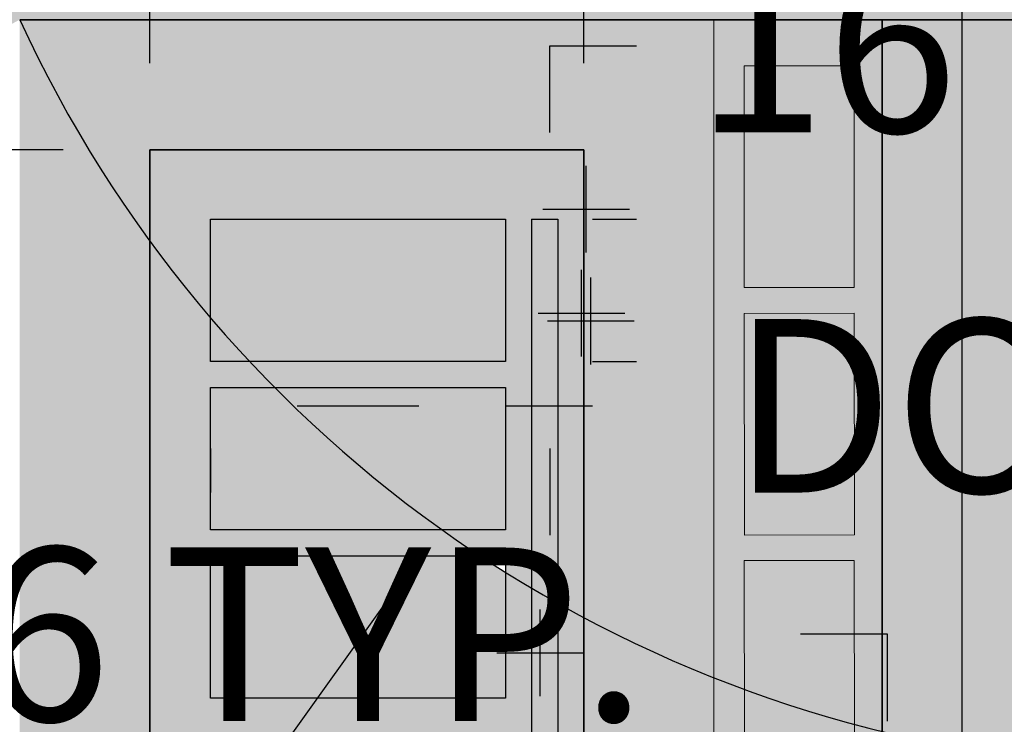
# Model space of a CAD drawing. Units: millimetres. Extents: x 130 to 1021, y 147 to 699.
# Tile 5 of 40: x 367 to 481, y 313 to 394. Entities that reach past the tile are written whole.
import ezdxf

# ---------------------------------------------------------------- set-up
doc = ezdxf.new("R2010")
doc.units = ezdxf.units.MM
doc.header["$MEASUREMENT"] = 0
for name, color, linetype, lineweight in [('A-ANNO-DIMS', 2, 'Continuous', 18), ('A-DOOR', 3, 'Continuous', 25), ('A-ELEV', 7, 'Continuous', 35), ('A-ELEV-PATT', 9, 'Continuous', 13), ('A-GLAZ', 4, 'Continuous', 18)]:
    doc.layers.add(name, color=color, linetype=linetype, lineweight=lineweight)
doc.styles.get("Standard").update_dxf_attribs({"font": 'arial.ttf'})
doc.dimstyles.get("Standard").update_dxf_attribs({"dimtxt": 20, "dimasz": 10, "dimexe": 10, "dimexo": 10, "dimgap": 5, "dimtad": 0, "dimtih": 1, "dimtoh": 1, "dimdec": 0, "dimzin": 0, "dimdsep": 46, "dimtxsty": 'Standard', "dimcen": 5, "dimadec": 0, "dimazin": 0, "dimtfac": 1, "dimtdec": 0, "dimtofl": 0, "dimtmove": 0, "dimatfit": 3, "dimfxl": 1, "dimtolj": 1, "dimtzin": 0, "dimarcsym": 0})

# ---------------------------------------------------------------- blocks, each defined once
blk = doc.blocks.new('DOOR-PANEL')
for p, q in [((0, 16.4), (34, 16.4)), ((0, 0), (0, 16.4)), ((34, 16.4), (34, 0)), ((34, 0), (0, 0))]:
    blk.add_line(p, q)
blk = doc.blocks.new('WIN-SIDELIGHT-PANE')
for p, q in [((0, 25.55), (12.68, 25.55)), ((0, 0), (0, 25.55)), ((12.68, 25.55), (12.68, 0)), ((12.68, 0), (0, 0))]:
    blk.add_line(p, q)
blk = doc.blocks.new('*D7')
at = {"layer": 'A-ANNO-DIMS', "color": 0, "lineweight": -2, "transparency": 16777216}
for p, q in [((399.37, 349.45), (413.37, 349.45)), ((423.37, 349.45), (433.37, 349.45)), ((389.37, 344.55), (389.37, 339.45)), ((423.37, 344.55), (423.37, 339.45))]:
    blk.add_line(p, q, dxfattribs=at)
at = {"layer": 'A-ANNO-DIMS', "color": 0, "transparency": 16777216}
for points in [[(399.37, 351.11), (399.37, 347.78), (389.37, 349.45)], [(413.37, 351.11), (413.37, 347.78), (423.37, 349.45)]]:
    blk.add_solid(points, dxfattribs=at)
at = {"layer": 'Defpoints', "color": 0, "transparency": 16777216}
for p in [(389.37, 354.55), (423.37, 354.55), (423.37, 349.45)]:
    blk.add_point(p, dxfattribs=at)
at = {"layer": 'A-ANNO-DIMS', "color": 0, "transparency": 16777216, "insert": (582.04, 349.45), "char_height": 20, "attachment_point": 5}
blk.add_mtext('\\A1;DOOR PANEL 34 TYP.', dxfattribs=at)
blk = doc.blocks.new('*D8')
at = {"layer": 'A-ANNO-DIMS', "color": 0, "lineweight": -2, "transparency": 16777216}
for p, q in [((428.47, 380.95), (428.47, 390.95)), ((428.47, 390.95), (438.47, 390.95)), ((433.37, 370.95), (438.47, 370.95)), ((433.37, 354.55), (438.47, 354.55)), ((428.47, 344.55), (428.47, 334.55))]:
    blk.add_line(p, q, dxfattribs=at)
at = {"layer": 'A-ANNO-DIMS', "color": 0, "transparency": 16777216}
for points in [[(426.81, 380.95), (430.14, 380.95), (428.47, 370.95)], [(426.81, 344.55), (430.14, 344.55), (428.47, 354.55)]]:
    blk.add_solid(points, dxfattribs=at)
at = {"layer": 'Defpoints', "color": 0, "transparency": 16777216}
for p in [(423.37, 370.95), (428.47, 370.95), (423.37, 354.55)]:
    blk.add_point(p, dxfattribs=at)
at = {"layer": 'A-ANNO-DIMS', "color": 0, "transparency": 16777216, "insert": (491.21, 390.95), "char_height": 20, "attachment_point": 5}
blk.add_mtext('\\A1;16 TYP.', dxfattribs=at)
blk = doc.blocks.new('*D9')
at = {"layer": 'A-ANNO-DIMS', "color": 0, "lineweight": -2, "transparency": 16777216}
for p, q in [((467.37, 323.13), (457.37, 323.13)), ((467.37, 313.13), (467.37, 323.13)), ((473.55, 303.13), (477.38, 303.13)), ((473.57, 277.58), (477.4, 277.58)), ((467.41, 267.57), (467.42, 257.57))]:
    blk.add_line(p, q, dxfattribs=at)
at = {"layer": 'A-ANNO-DIMS', "color": 0, "transparency": 16777216}
for points in [[(469.04, 313.13), (465.71, 313.13), (467.38, 303.13)], [(469.08, 267.57), (465.75, 267.57), (467.4, 277.57)]]:
    blk.add_solid(points, dxfattribs=at)
at = {"layer": 'Defpoints', "color": 0, "transparency": 16777216}
for p in [(463.55, 303.12), (467.38, 303.13), (463.57, 277.57)]:
    blk.add_point(p, dxfattribs=at)
at = {"layer": 'A-ANNO-DIMS', "color": 0, "transparency": 16777216, "insert": (284.19, 323.13), "char_height": 20, "attachment_point": 5}
blk.add_mtext('\\A1;SIDELIGHT PANE 26 TYP.', dxfattribs=at)
blk = doc.blocks.new('*D11')
at = {"layer": 'A-ANNO-DIMS', "color": 0, "lineweight": -2, "transparency": 16777216}
for p, q in [((737.37, 648.7), (737.37, 149.74)), ((299.37, 566.95), (299.37, 149.74)), ((309.37, 159.74), (490.86, 159.74)), ((727.37, 159.74), (545.89, 159.74))]:
    blk.add_line(p, q, dxfattribs=at)
at = {"layer": 'A-ANNO-DIMS', "color": 0, "transparency": 16777216}
for points in [[(309.37, 161.41), (309.37, 158.07), (299.37, 159.74)], [(727.37, 161.41), (727.37, 158.07), (737.37, 159.74)]]:
    blk.add_solid(points, dxfattribs=at)
at = {"layer": 'Defpoints', "color": 0, "transparency": 16777216}
for p in [(737.37, 658.7), (299.37, 576.95), (737.37, 159.74)]:
    blk.add_point(p, dxfattribs=at)
at = {"layer": 'A-ANNO-DIMS', "color": 0, "transparency": 16777216, "insert": (518.37, 159.74), "char_height": 20, "attachment_point": 5}
blk.add_mtext('\\A1;438', dxfattribs=at)
blk = doc.blocks.new('*D12')
at = {"layer": 'A-ANNO-DIMS', "color": 0, "lineweight": -2, "transparency": 16777216}
for p, q in [((477.37, 661.95), (265.07, 661.95)), ((275.07, 651.95), (275.07, 438.2)), ((275.07, 194.04), (275.07, 407.78)), ((357.16, 184.04), (265.07, 184.04))]:
    blk.add_line(p, q, dxfattribs=at)
at = {"layer": 'A-ANNO-DIMS', "color": 0, "transparency": 16777216}
for points in [[(273.41, 651.95), (276.74, 651.95), (275.07, 661.95)], [(273.41, 194.04), (276.74, 194.04), (275.07, 184.04)]]:
    blk.add_solid(points, dxfattribs=at)
at = {"layer": 'Defpoints', "color": 0, "transparency": 16777216}
for p in [(275.07, 661.95), (487.37, 661.95), (367.16, 184.04)]:
    blk.add_point(p, dxfattribs=at)
at = {"layer": 'A-ANNO-DIMS', "color": 0, "transparency": 16777216, "insert": (275.07, 422.99), "char_height": 20, "attachment_point": 5}
blk.add_mtext('\\A1;477.9', dxfattribs=at)
blk = doc.blocks.new('*D18')
at = {"layer": 'A-ANNO-DIMS', "color": 0, "lineweight": -2, "transparency": 16777216}
for p, q in [((375.85, 490.22), (375.85, 696.25)), ((382.37, 388.95), (382.37, 696.25)), ((365.85, 686.25), (355.85, 686.25)), ((392.37, 686.25), (402.37, 686.25))]:
    blk.add_line(p, q, dxfattribs=at)
at = {"layer": 'A-ANNO-DIMS', "color": 0, "transparency": 16777216}
for points in [[(365.85, 687.91), (365.85, 684.58), (375.85, 686.25)], [(392.37, 687.91), (392.37, 684.58), (382.37, 686.25)]]:
    blk.add_solid(points, dxfattribs=at)
at = {"layer": 'Defpoints', "color": 0, "transparency": 16777216}
for p in [(382.37, 686.25), (375.85, 480.22), (382.37, 378.95)]:
    blk.add_point(p, dxfattribs=at)
at = {"layer": 'A-ANNO-DIMS', "color": 0, "transparency": 16777216, "insert": (441.13, 686.25), "char_height": 20, "attachment_point": 5}
blk.add_mtext('\\A1;6.524', dxfattribs=at)
blk = doc.blocks.new('*D19')
at = {"layer": 'A-ANNO-DIMS', "color": 0, "lineweight": -2, "transparency": 16777216}
for p, q in [((382.37, 388.95), (382.37, 696.25)), ((414.65, 510.88), (414.65, 696.25)), ((392.37, 686.25), (404.65, 686.25)), ((414.65, 686.25), (424.65, 686.25))]:
    blk.add_line(p, q, dxfattribs=at)
at = {"layer": 'A-ANNO-DIMS', "color": 0, "transparency": 16777216}
for points in [[(392.37, 687.91), (392.37, 684.58), (382.37, 686.25)], [(404.65, 687.91), (404.65, 684.58), (414.65, 686.25)]]:
    blk.add_solid(points, dxfattribs=at)
at = {"layer": 'Defpoints', "color": 0, "transparency": 16777216}
for p in [(414.65, 686.25), (414.65, 500.88), (382.37, 378.95)]:
    blk.add_point(p, dxfattribs=at)
at = {"layer": 'A-ANNO-DIMS', "color": 0, "transparency": 16777216, "insert": (463.41, 686.25), "char_height": 20, "attachment_point": 5}
blk.add_mtext('\\A1;32.28', dxfattribs=at)
blk = doc.blocks.new('*D20')
at = {"layer": 'A-ANNO-DIMS', "color": 0, "lineweight": -2, "transparency": 16777216}
for p, q in [((414.65, 510.88), (414.65, 696.25)), ((432.37, 388.95), (432.37, 696.25)), ((404.65, 686.25), (394.65, 686.25)), ((442.37, 686.25), (452.37, 686.25))]:
    blk.add_line(p, q, dxfattribs=at)
at = {"layer": 'A-ANNO-DIMS', "color": 0, "transparency": 16777216}
for points in [[(404.65, 687.91), (404.65, 684.58), (414.65, 686.25)], [(442.37, 687.91), (442.37, 684.58), (432.37, 686.25)]]:
    blk.add_solid(points, dxfattribs=at)
at = {"layer": 'Defpoints', "color": 0, "transparency": 16777216}
for p in [(432.37, 686.25), (414.65, 500.88), (432.37, 378.95)]:
    blk.add_point(p, dxfattribs=at)
at = {"layer": 'A-ANNO-DIMS', "color": 0, "transparency": 16777216, "insert": (490.08, 686.25), "char_height": 20, "attachment_point": 5}
blk.add_mtext('\\A1;17.72', dxfattribs=at)
blk = doc.blocks.new('*D21')
at = {"layer": 'A-ANNO-DIMS', "color": 0, "lineweight": -2, "transparency": 16777216}
for p, q in [((432.37, 388.95), (432.37, 696.25)), ((447.37, 656.95), (447.37, 696.25)), ((422.37, 686.25), (412.37, 686.25)), ((457.37, 686.25), (467.37, 686.25))]:
    blk.add_line(p, q, dxfattribs=at)
at = {"layer": 'A-ANNO-DIMS', "color": 0, "transparency": 16777216}
for points in [[(422.37, 687.91), (422.37, 684.58), (432.37, 686.25)], [(457.37, 687.91), (457.37, 684.58), (447.37, 686.25)]]:
    blk.add_solid(points, dxfattribs=at)
at = {"layer": 'Defpoints', "color": 0, "transparency": 16777216}
for p in [(447.37, 686.25), (447.37, 646.95), (432.37, 378.95)]:
    blk.add_point(p, dxfattribs=at)
at = {"layer": 'A-ANNO-DIMS', "color": 0, "transparency": 16777216, "insert": (485.83, 686.25), "char_height": 20, "attachment_point": 5}
blk.add_mtext('\\A1;15', dxfattribs=at)
blk = doc.blocks.new('*D23')
at = {"layer": 'A-ANNO-DIMS', "color": 0, "lineweight": -2, "transparency": 16777216}
for p, q in [((466.77, 403.95), (466.77, 696.25)), ((475.99, 209.04), (475.99, 696.25)), ((456.77, 686.25), (446.77, 686.25)), ((485.99, 686.25), (495.99, 686.25))]:
    blk.add_line(p, q, dxfattribs=at)
at = {"layer": 'A-ANNO-DIMS', "color": 0, "transparency": 16777216}
for points in [[(456.77, 687.91), (456.77, 684.58), (466.77, 686.25)], [(485.99, 687.91), (485.99, 684.58), (475.99, 686.25)]]:
    blk.add_solid(points, dxfattribs=at)
at = {"layer": 'Defpoints', "color": 0, "transparency": 16777216}
for p in [(475.99, 686.25), (466.77, 393.95), (475.99, 199.04)]:
    blk.add_point(p, dxfattribs=at)
at = {"layer": 'A-ANNO-DIMS', "color": 0, "transparency": 16777216, "insert": (534.63, 686.25), "char_height": 20, "attachment_point": 5}
blk.add_mtext('\\A1;9.222', dxfattribs=at)
blk = doc.blocks.new('*D24')
at = {"layer": 'A-ANNO-DIMS', "color": 0, "lineweight": -2, "transparency": 16777216}
for p, q in [((475.99, 209.04), (475.99, 696.25)), ((487.37, 671.95), (487.37, 696.25)), ((465.99, 686.25), (455.99, 686.25)), ((497.37, 686.25), (507.37, 686.25))]:
    blk.add_line(p, q, dxfattribs=at)
at = {"layer": 'A-ANNO-DIMS', "color": 0, "transparency": 16777216}
for points in [[(465.99, 687.91), (465.99, 684.58), (475.99, 686.25)], [(497.37, 687.91), (497.37, 684.58), (487.37, 686.25)]]:
    blk.add_solid(points, dxfattribs=at)
at = {"layer": 'Defpoints', "color": 0, "transparency": 16777216}
for p in [(487.37, 686.25), (487.37, 661.95), (475.99, 199.04)]:
    blk.add_point(p, dxfattribs=at)
at = {"layer": 'A-ANNO-DIMS', "color": 0, "transparency": 16777216, "insert": (553.02, 686.25), "char_height": 20, "attachment_point": 5}
blk.add_mtext('\\A1;11.385', dxfattribs=at)
blk = doc.blocks.new('*D60')
at = {"layer": 'A-ANNO-DIMS', "color": 0, "lineweight": -2, "transparency": 16777216}
for p, q in [((372.37, 378.95), (265.07, 378.95)), ((275.07, 368.95), (275.07, 329.46)), ((275.07, 259.55), (275.07, 299.04)), ((372.37, 249.55), (265.07, 249.55))]:
    blk.add_line(p, q, dxfattribs=at)
at = {"layer": 'A-ANNO-DIMS', "color": 0, "transparency": 16777216}
for points in [[(273.41, 368.95), (276.74, 368.95), (275.07, 378.95)], [(273.41, 259.55), (276.74, 259.55), (275.07, 249.55)]]:
    blk.add_solid(points, dxfattribs=at)
at = {"layer": 'Defpoints', "color": 0, "transparency": 16777216}
for p in [(275.07, 378.95), (382.37, 378.95), (382.37, 249.55)]:
    blk.add_point(p, dxfattribs=at)
at = {"layer": 'A-ANNO-DIMS', "color": 0, "transparency": 16777216, "insert": (275.07, 314.25), "char_height": 20, "attachment_point": 5}
blk.add_mtext('\\A1;129.4', dxfattribs=at)
blk = doc.blocks.new('*D64')
at = {"layer": 'A-ANNO-DIMS', "color": 0, "lineweight": -2, "transparency": 16777216}
for p, q in [((502.05, 450.93), (502.05, 460.93)), ((497.05, 455.93), (507.05, 455.93)), ((363.96, 263.06), (409.92, 327.25)), ((353.96, 263.06), (363.96, 263.06))]:
    blk.add_line(p, q, dxfattribs=at)
at = {"layer": 'A-ANNO-DIMS', "color": 0, "transparency": 16777216}
blk.add_solid([(408.57, 328.22), (411.28, 326.28), (415.74, 335.39)], dxfattribs=at)
at = {"layer": 'Defpoints', "color": 0, "transparency": 16777216}
for p in [(502.05, 455.93), (415.74, 335.39)]:
    blk.add_point(p, dxfattribs=at)
at = {"layer": 'A-ANNO-DIMS', "color": 0, "transparency": 16777216, "insert": (297.8, 263.06), "char_height": 20, "attachment_point": 5}
blk.add_mtext('\\A1;R148.25', dxfattribs=at)
blk = doc.blocks.new('*D65')
at = {"layer": 'A-ANNO-DIMS', "color": 0, "lineweight": -2, "transparency": 16777216}
for p, q in [((495.46, 509.13), (472.51, 423.11)), ((505.46, 509.13), (495.46, 509.13)), ((427.37, 248.98), (427.37, 258.98)), ((422.37, 253.98), (432.37, 253.98))]:
    blk.add_line(p, q, dxfattribs=at)
at = {"layer": 'A-ANNO-DIMS', "color": 0, "transparency": 16777216}
blk.add_solid([(470.9, 423.54), (474.12, 422.68), (469.93, 413.45)], dxfattribs=at)
at = {"layer": 'Defpoints', "color": 0, "transparency": 16777216}
for p in [(469.93, 413.45), (427.37, 253.98)]:
    blk.add_point(p, dxfattribs=at)
at = {"layer": 'A-ANNO-DIMS', "color": 0, "transparency": 16777216, "insert": (561.62, 509.13), "char_height": 20, "attachment_point": 5}
blk.add_mtext('\\A1;R165.05', dxfattribs=at)
blk = doc.blocks.new('*D66')
at = {"layer": 'A-ANNO-DIMS', "color": 0, "lineweight": -2, "transparency": 16777216}
for p, q in [((341.58, 557.19), (351.58, 557.19)), ((351.58, 557.19), (376.95, 478.14)), ((427.37, 315.98), (427.37, 325.98)), ((422.37, 320.98), (432.37, 320.98))]:
    blk.add_line(p, q, dxfattribs=at)
at = {"layer": 'A-ANNO-DIMS', "color": 0, "transparency": 16777216}
blk.add_solid([(378.53, 478.64), (375.36, 477.63), (380, 468.61)], dxfattribs=at)
at = {"layer": 'Defpoints', "color": 0, "transparency": 16777216}
for p in [(380, 468.61), (427.37, 320.98)]:
    blk.add_point(p, dxfattribs=at)
at = {"layer": 'A-ANNO-DIMS', "color": 0, "transparency": 16777216, "insert": (263.53, 557.19), "char_height": 20, "attachment_point": 5}
blk.add_mtext('\\A1;4X R155.05', dxfattribs=at)
blk = doc.blocks.new('*D67')
at = {"layer": 'A-ANNO-DIMS', "color": 0, "lineweight": -2, "transparency": 16777216}
for p, q in [((479.76, 492.43), (462.14, 412.22)), ((489.76, 492.43), (479.76, 492.43)), ((427.07, 247.5), (427.07, 257.5)), ((422.07, 252.5), (432.07, 252.5))]:
    blk.add_line(p, q, dxfattribs=at)
at = {"layer": 'A-ANNO-DIMS', "color": 0, "transparency": 16777216}
blk.add_solid([(460.52, 412.58), (463.77, 411.87), (460, 402.46)], dxfattribs=at)
at = {"layer": 'Defpoints', "color": 0, "transparency": 16777216}
for p in [(460, 402.46), (427.07, 252.5)]:
    blk.add_point(p, dxfattribs=at)
at = {"layer": 'A-ANNO-DIMS', "color": 0, "transparency": 16777216, "insert": (545.84, 492.43), "char_height": 20, "attachment_point": 5}
blk.add_mtext('\\A1;R153.53', dxfattribs=at)
blk = doc.blocks.new('*D68')
at = {"layer": 'A-ANNO-DIMS', "color": 0, "lineweight": -2, "transparency": 16777216}
for p, q in [((361.84, 579.76), (371.84, 579.76)), ((371.84, 579.76), (392.17, 506.69)), ((433.19, 354.23), (433.19, 364.23)), ((428.19, 359.23), (438.19, 359.23))]:
    blk.add_line(p, q, dxfattribs=at)
at = {"layer": 'A-ANNO-DIMS', "color": 0, "transparency": 16777216}
blk.add_solid([(393.77, 507.14), (390.56, 506.25), (394.85, 497.06)], dxfattribs=at)
at = {"layer": 'Defpoints', "color": 0, "transparency": 16777216}
for p in [(394.85, 497.06), (433.19, 359.23)]:
    blk.add_point(p, dxfattribs=at)
at = {"layer": 'A-ANNO-DIMS', "color": 0, "transparency": 16777216, "insert": (305.76, 579.76), "char_height": 20, "attachment_point": 5}
blk.add_mtext('\\A1;R143.06', dxfattribs=at)
blk = doc.blocks.new('*D69')
at = {"layer": 'A-ANNO-DIMS', "color": 0, "lineweight": -2, "transparency": 16777216}
for p, q in [((507.75, 572.26), (483.09, 501.81)), ((517.75, 572.26), (507.75, 572.26)), ((433.19, 354.23), (433.19, 364.23)), ((428.19, 359.23), (438.19, 359.23))]:
    blk.add_line(p, q, dxfattribs=at)
at = {"layer": 'A-ANNO-DIMS', "color": 0, "transparency": 16777216}
blk.add_solid([(481.52, 502.36), (484.66, 501.26), (479.79, 492.37)], dxfattribs=at)
at = {"layer": 'Defpoints', "color": 0, "transparency": 16777216}
for p in [(479.79, 492.37), (433.19, 359.23)]:
    blk.add_point(p, dxfattribs=at)
at = {"layer": 'A-ANNO-DIMS', "color": 0, "transparency": 16777216, "insert": (573.82, 572.26), "char_height": 20, "attachment_point": 5}
blk.add_mtext('\\A1;R141.06', dxfattribs=at)
blk = doc.blocks.new('*D70')
at = {"layer": 'A-ANNO-DIMS', "color": 0, "lineweight": -2, "transparency": 16777216}
for p, q in [((370.14, 588.4), (380.14, 588.4)), ((380.14, 588.4), (397.47, 517.01)), ((432.65, 367.11), (432.65, 377.11)), ((427.65, 372.11), (437.65, 372.11))]:
    blk.add_line(p, q, dxfattribs=at)
at = {"layer": 'A-ANNO-DIMS', "color": 0, "transparency": 16777216}
blk.add_solid([(399.09, 517.4), (395.85, 516.62), (399.83, 507.29)], dxfattribs=at)
at = {"layer": 'Defpoints', "color": 0, "transparency": 16777216}
for p in [(399.83, 507.29), (432.65, 372.11)]:
    blk.add_point(p, dxfattribs=at)
at = {"layer": 'A-ANNO-DIMS', "color": 0, "transparency": 16777216, "insert": (323.76, 588.4), "char_height": 20, "attachment_point": 5}
blk.add_mtext('\\A1;R139.1', dxfattribs=at)
blk = doc.blocks.new('*D71')
at = {"layer": 'A-ANNO-DIMS', "color": 0, "lineweight": -2, "transparency": 16777216}
for p, q in [((492.11, 581.61), (472.54, 512.67)), ((502.11, 581.61), (492.11, 581.61)), ((432.65, 367.11), (432.65, 377.11)), ((427.65, 372.11), (437.65, 372.11))]:
    blk.add_line(p, q, dxfattribs=at)
at = {"layer": 'A-ANNO-DIMS', "color": 0, "transparency": 16777216}
blk.add_solid([(470.94, 513.12), (474.15, 512.21), (469.81, 503.05)], dxfattribs=at)
at = {"layer": 'Defpoints', "color": 0, "transparency": 16777216}
for p in [(469.81, 503.05), (432.65, 372.11)]:
    blk.add_point(p, dxfattribs=at)
at = {"layer": 'A-ANNO-DIMS', "color": 0, "transparency": 16777216, "insert": (548.49, 581.61), "char_height": 20, "attachment_point": 5}
blk.add_mtext('\\A1;R136.1', dxfattribs=at)
blk = doc.blocks.new('*D72')
at = {"layer": 'A-ANNO-DIMS', "color": 0, "lineweight": -2, "transparency": 16777216}
for p, q in [((460.66, 573.64), (451.28, 503.49)), ((470.66, 573.64), (460.66, 573.64)), ((432.11, 355.14), (432.11, 365.14)), ((427.11, 360.14), (437.11, 360.14))]:
    blk.add_line(p, q, dxfattribs=at)
at = {"layer": 'A-ANNO-DIMS', "color": 0, "transparency": 16777216}
blk.add_solid([(449.63, 503.71), (452.93, 503.27), (449.95, 493.58)], dxfattribs=at)
at = {"layer": 'Defpoints', "color": 0, "transparency": 16777216}
for p in [(449.95, 493.58), (432.11, 360.14)]:
    blk.add_point(p, dxfattribs=at)
at = {"layer": 'A-ANNO-DIMS', "color": 0, "transparency": 16777216, "insert": (526.64, 573.64), "char_height": 20, "attachment_point": 5}
blk.add_mtext('\\A1;R134.62', dxfattribs=at)
blk = doc.blocks.new('*D73')
at = {"layer": 'A-ANNO-DIMS', "color": 0, "lineweight": -2, "transparency": 16777216}
for p, q in [((402.68, 571.45), (412.68, 571.45)), ((412.68, 571.45), (419.05, 502.17)), ((432.11, 355.14), (432.11, 365.14)), ((427.11, 360.14), (437.11, 360.14))]:
    blk.add_line(p, q, dxfattribs=at)
at = {"layer": 'A-ANNO-DIMS', "color": 0, "transparency": 16777216}
blk.add_solid([(420.71, 502.32), (417.39, 502.01), (419.97, 492.21)], dxfattribs=at)
at = {"layer": 'Defpoints', "color": 0, "transparency": 16777216}
for p in [(419.97, 492.21), (432.11, 360.14)]:
    blk.add_point(p, dxfattribs=at)
at = {"layer": 'A-ANNO-DIMS', "color": 0, "transparency": 16777216, "insert": (346.7, 571.45), "char_height": 20, "attachment_point": 5}
blk.add_mtext('\\A1;R132.62', dxfattribs=at)

msp = doc.modelspace()

# ---------------------------------------------------------------- hatches: boundary and pattern name
at = {"layer": 'A-ELEV-PATT'}
h = msp.add_hatch(color=256, dxfattribs=at)
h.dxf.hatch_style = 1
h.paths.add_polyline_path([(447.3738, 576.9473), (302.3738, 576.9473), (302.3738, 573.9473), (447.3738, 573.9473)])
h.paths.add_polyline_path([(487.3738, 583.9473), (487.3738, 586.9473), (447.3738, 576.9473), (447.3738, 573.9473)])
h.paths.add_polyline_path([(632.355, 586.9473), (487.3738, 586.9473), (487.3738, 583.9473), (632.3738, 583.9473), (632.3738, 583.9472, -0.01380003), (737.3738, 580.6507), (737.3738, 583.6559, 0.01378075)])
h.paths.add_polyline_path([(367.3738, 466.9473), (302.3738, 466.9473), (302.3738, 463.9473), (367.3738, 463.9473)])
h.paths.add_polyline_path([(487.3738, 463.9473), (487.3738, 466.9473, 0.20133085), (367.3738, 466.9473), (367.3738, 463.9473, -0.20132998)])
h.paths.add_polyline_path([(632.3738, 466.9473), (487.3738, 466.9473), (487.3738, 463.9473), (632.3681, 463.9473, -0.01372855), (737.3738, 460.6681), (737.3738, 463.6732, 0.01370629)])
h.paths.add_polyline_path([(632.3738, 396.9473), (487.3738, 396.9473, 0.20133085), (367.3738, 396.9473), (367.3738, 393.9473, -0.20237172), (486.7667, 393.9473), (632.3681, 393.9473, -0.01372855), (737.3738, 390.6681), (737.3738, 393.6732, 0.01370629)])
h.paths.add_polyline_path([(357.9413, 391.9473), (307.3738, 391.9473), (307.3738, 388.9473), (357.9413, 388.9473)])
h.paths.add_polyline_path([(367.3738, 393.9473), (367.3738, 396.9473), (357.9413, 391.924), (357.9413, 388.9473), (358.058, 388.9473)])
h.paths.add_polyline_path([(737.3738, 264.2162), (737.3738, 267.2214, -0.01370629), (632.3738, 263.9473), (463.7667, 263.9473), (466.7667, 260.9473), (632.3794, 260.9473, 0.01368411)])
h.paths.add_polyline_path([(463.7667, 263.9473), (447.3738, 263.9473), (450.3738, 260.9473), (466.7667, 260.9473)])
h.paths.add_polyline_path([(447.3738, 263.9473), (432.3738, 263.9473), (432.3738, 260.9473), (450.3738, 260.9473)])
h.paths.add_polyline_path([(382.3738, 263.9473), (357.9413, 263.9473), (357.9413, 260.9473), (382.3738, 260.9473)])
h.paths.add_polyline_path([(357.9413, 263.9473), (307.3738, 263.9473), (307.3738, 260.9473), (357.9413, 260.9473)])
h = msp.add_hatch(color=256, dxfattribs=at)
h.paths.add_polyline_path([(327.3738, 569.884), (327.3738, 573.9473), (307.3738, 573.9473), (307.3738, 476.9473), (327.3738, 476.9473), (327.3738, 480.95)])
h.paths.add_polyline_path([(486.7667, 386.2639), (486.7667, 393.9473), (466.7667, 393.9473), (466.7667, 357.2114), (466.7667, 311.9335, 0.03427026), (486.7667, 308.4637)])
h.paths.add_polyline_path([(486.7667, 308.4637, -0.03427026), (466.7667, 311.9335), (466.7667, 273.9473), (486.7667, 273.9473)])
h.paths.add_polyline_path([(389.3738, 351.5473), (396.7693, 351.5473, -0.00702703), (393.8774, 354.5473), (389.3738, 354.5473), (389.3738, 359.5775, -0.01903024), (382.3738, 368.424), (382.3738, 249.5473), (432.3738, 249.5473), (432.3738, 325.067, -0.00576734), (429.3738, 326.709), (429.3738, 257.5473), (426.3738, 257.5473), (426.3738, 328.4428, -0.00592542), (423.3738, 330.272), (423.3738, 315.7473), (389.3738, 315.7473), (389.3738, 332.1473), (420.4552, 332.1473, -0.00895099), (416.0768, 335.1473), (389.3738, 335.1473)])
h.paths.add_polyline_path([(389.3738, 312.7473), (423.3738, 312.7473), (423.3738, 296.3473), (389.3738, 296.3473)], flags=16)
h.paths.add_polyline_path([(389.3738, 293.3473), (423.3738, 293.3473), (423.3738, 276.9473), (389.3738, 276.9473)], flags=16)
h.paths.add_polyline_path([(389.3738, 273.9473), (423.3738, 273.9473), (423.3738, 257.5473), (389.3738, 257.5473)], flags=16)
h.paths.add_polyline_path([(432.3738, 378.9473), (382.3738, 378.9473), (382.3738, 368.424, 0.01903024), (389.3738, 359.5775), (389.3738, 370.9473), (423.3738, 370.9473), (423.3738, 354.5473), (393.8774, 354.5473, 0.00702703), (396.7693, 351.5473), (423.3738, 351.5473), (423.3738, 335.1473), (416.0768, 335.1473, 0.00895099), (420.4552, 332.1473), (423.3738, 332.1473), (423.3738, 330.272, 0.00592542), (426.3738, 328.4428), (426.3738, 370.9473), (429.3738, 370.9473), (429.3738, 326.709, 0.00576734), (432.3738, 325.067)])
h.paths.add_polyline_path([(466.7667, 357.2114), (466.7667, 393.9473), (447.3738, 393.9473), (447.3738, 357.2114), (447.3738, 318.1243, 0.0063261), (450.8779, 316.785), (450.8779, 331.5915), (463.5608, 331.5915), (463.5608, 312.7571, 0.00558197), (466.7667, 311.9335)])
h.paths.add_polyline_path([(450.8779, 334.5915), (450.8779, 360.0915), (463.5608, 360.0915), (463.5608, 334.5915)], flags=16)
h.paths.add_polyline_path([(450.8779, 363.0915), (450.8779, 388.6449), (463.5608, 388.6449), (463.5608, 363.0915)], flags=16)
h.paths.add_polyline_path([(466.7667, 311.9335, -0.00558197), (463.5608, 312.7571), (463.5608, 306.0915), (450.8779, 306.0915), (450.8779, 316.785, -0.0063261), (447.3738, 318.1243), (447.3738, 273.9473), (466.7667, 273.9473)])
h.paths.add_polyline_path([(450.8779, 303.0915), (463.5608, 303.0915), (463.5608, 277.5915), (450.8779, 277.5915)], flags=16)
h.paths.add_polyline_path([(552.3738, 357.2114), (552.3738, 393.9473), (486.7667, 393.9473), (486.7667, 386.2639), (544.6354, 386.2639), (544.6354, 280.6619), (486.7667, 280.6619), (486.7667, 273.9473), (552.3738, 273.9473)])
h.paths.add_polyline_path([(487.3738, 583.9473), (472.3738, 580.1973), (472.3738, 507.0765), (472.3738, 505.4251, -0.00564525), (475.3738, 504.4942), (475.3738, 506.3543), (475.3738, 511.9473), (484.3738, 511.9473), (484.3738, 503.8134), (484.3738, 501.2439, -0.00583574), (487.3738, 500.0015)])
h.paths.add_polyline_path([(484.3738, 578.0434), (484.3738, 548.9473), (475.3738, 548.9473), (475.3738, 575.7934)], flags=16)
h.paths.add_polyline_path([(484.3738, 546.9473), (484.3738, 513.9473), (475.3738, 513.9473), (475.3738, 518.7148), (475.3738, 546.9473)], flags=16)
h = msp.add_hatch(color=256, dxfattribs=at)
h.dxf.hatch_style = 1
h.paths.add_polyline_path([(363.922, 569.884), (327.3738, 569.884), (327.3738, 557.9168), (363.922, 557.9168)])
h.paths.add_polyline_path([(547.7773, 577.3739), (502.3738, 577.3739), (502.3738, 566.2111), (547.7773, 566.2111)])
h.paths.add_polyline_path([(544.6354, 386.2639), (486.7667, 386.2639), (486.7667, 377.43), (544.6354, 377.43)])
h.paths.add_polyline_path([(496.0546, 377.43), (486.7667, 377.43), (486.7667, 370.4028)])
h.paths.add_polyline_path([(447.3738, 393.9473), (367.3738, 393.9473, 0.05004781), (382.3738, 368.424), (382.3738, 378.9473), (432.3738, 378.9473), (432.3738, 325.067, 0.02789446), (447.3738, 318.1243), (447.3738, 357.2114)])
h.paths.add_polyline_path([(463.5608, 388.6449), (450.8779, 388.6449), (450.8779, 363.0915), (463.5608, 363.0915)])
h.paths.add_polyline_path([(463.5608, 360.0915), (450.8779, 360.0915), (450.8779, 334.5915), (463.5608, 334.5915)])
h.paths.add_polyline_path([(463.5608, 331.5915), (450.8779, 331.5915), (450.8779, 316.785, 0.02245133), (463.5608, 312.7571)])
msp.add_hatch(color=256, dxfattribs=at).paths.add_polyline_path([(367.3738, 393.9473), (486.7667, 393.9473, 0.20237172)])
h = msp.add_hatch(color=256, dxfattribs=at)
h.dxf.hatch_style = 1
h.paths.add_polyline_path([(382.3738, 368.424, -0.05004781), (367.3738, 393.9473), (367.3738, 357.2114), (367.3738, 273.9473), (382.3738, 273.9473)])
h.paths.add_polyline_path([(432.3738, 273.9473), (447.3738, 273.9473), (447.3738, 318.1243, -0.02789446), (432.3738, 325.067)])
h.paths.add_polyline_path([(463.5608, 306.0915), (463.5608, 312.7571, -0.02245133), (450.8779, 316.785), (450.8779, 306.0915)])
h.paths.add_polyline_path([(450.8779, 303.0915), (450.8779, 277.5915), (463.5608, 277.5915), (463.5608, 303.0915)])
h = msp.add_hatch(color=256, dxfattribs=at)
h.set_gradient(color1=(221, 197, 207), color2=(86, 84, 89), name='CURVED')
h.paths.add_polyline_path([(423.3738, 273.9473), (389.3738, 273.9473), (389.3738, 257.5473), (423.3738, 257.5473)])
h.paths.add_polyline_path([(423.3738, 293.3473), (389.3738, 293.3473), (389.3738, 276.9473), (423.3738, 276.9473)])
h.paths.add_polyline_path([(423.3738, 312.7473), (389.3738, 312.7473), (389.3738, 296.3473), (423.3738, 296.3473)])
h.paths.add_polyline_path([(423.3738, 330.272, -0.00585023), (420.4552, 332.1473), (389.3738, 332.1473), (389.3738, 315.7473), (423.3738, 315.7473)])
h.paths.add_polyline_path([(396.7693, 351.5473), (389.3738, 351.5473), (389.3738, 335.1473), (416.0768, 335.1473, -0.04279691)])
h.paths.add_polyline_path([(423.3738, 351.5473), (396.7693, 351.5473, 0.04279691), (416.0768, 335.1473), (423.3738, 335.1473)])
h.paths.add_polyline_path([(423.3738, 370.9473), (389.3738, 370.9473), (389.3738, 359.5775, 0.01138691), (393.8774, 354.5473), (423.3738, 354.5473)])
h.paths.add_polyline_path([(389.3738, 359.5775), (389.3738, 354.5473), (393.8774, 354.5473, -0.01138691)], flags=17)
h = msp.add_hatch(color=256, dxfattribs=at)
h.set_gradient(color1=(221, 197, 207), color2=(86, 84, 89), name='CURVED')
h.paths.add_polyline_path([(429.3738, 326.709, -0.00584318), (426.3738, 328.4428), (426.3738, 257.5473), (429.3738, 257.5473)])
h.paths.add_polyline_path([(426.3738, 328.4428, 0.00584318), (429.3738, 326.709), (429.3738, 370.9473), (426.3738, 370.9473)])

# ---------------------------------------------------------------- linework, layer by layer
at = {"layer": 'A-DOOR'}
for p, q in [((426.3738, 370.9473), (429.3738, 370.9473)), ((426.3738, 370.9473), (426.3738, 257.5473)), ((429.3738, 370.9473), (429.3738, 257.5473))]:
    msp.add_line(p, q, dxfattribs=at)
msp.add_arc((502.0489, 455.9263), 148.2524, 204.712441, 264.083334, dxfattribs=at)
at = {"layer": 'A-ELEV'}
for p, q in [((632.3738, 393.9473), (367.3738, 393.9473)), ((466.7667, 393.9473), (466.7667, 357.2114)), ((382.3738, 378.9473), (432.3738, 378.9473)), ((382.3738, 249.5473), (382.3738, 378.9473)), ((432.3738, 378.9473), (432.3738, 249.5473)), ((466.7667, 357.2114), (466.7667, 273.9473))]:
    msp.add_line(p, q, dxfattribs=at)
at = {"layer": 'A-GLAZ'}
for p, q in [((447.3738, 393.9473), (447.3738, 357.2114)), ((447.3738, 357.2114), (447.3738, 273.9473))]:
    msp.add_line(p, q, dxfattribs=at)

# ---------------------------------------------------------------- block references
at = {"layer": 'A-DOOR'}
msp.add_blockref('DOOR-PANEL', (389.374, 354.547), dxfattribs=at)
at = {"layer": 'A-DOOR', "rotation": 180}
for p in [(423.3736, 351.5476), (423.3736, 332.1476)]:
    msp.add_blockref('DOOR-PANEL', p, dxfattribs=at)
at = {"layer": 'A-GLAZ'}
msp.add_blockref('WIN-SIDELIGHT-PANE', (450.878, 363.091), dxfattribs=at)
at = {"layer": 'A-GLAZ', "rotation": 0.0477534205481112}
for p in [(450.8887, 334.559), (450.8887, 306.059)]:
    msp.add_blockref('WIN-SIDELIGHT-PANE', p, dxfattribs=at)

# ---------------------------------------------------------------- dimensions: what is measured, and where the dimension line sits
at = {"layer": 'A-ANNO-DIMS'}
for base, p1, p2, override, picture, middle in [((382.3738, 686.2473), (375.8501, 480.2159), (382.3738, 378.9473), {"dimdec": 3, "dimlfac": 1, "dimrnd": 0, "dimzin": 0, "dimdsep": 46, "dimlunit": 2}, '*D18', (441.1323, 686.2473)), ((414.6525, 686.2473), (382.3738, 378.9473), (414.6525, 500.8811), {"dimdec": 2, "dimlfac": 1, "dimrnd": 0, "dimzin": 0, "dimdsep": 46, "dimlunit": 2}, '*D19', (463.411, 686.2473)), ((432.3738, 686.2473), (414.6525, 500.8811), (432.3738, 378.9473), {"dimdec": 2, "dimlfac": 1, "dimrnd": 0, "dimzin": 0, "dimdsep": 46, "dimlunit": 2}, '*D20', (490.075, 686.2473)), ((447.3738, 686.2473), (432.3738, 378.9473), (447.3738, 646.9473), {"dimdec": 0, "dimlfac": 1, "dimrnd": 0, "dimzin": 0, "dimdsep": 46, "dimlunit": 2}, '*D21', (485.8322, 686.2473)), ((475.9885, 686.2473), (466.7667, 393.9473), (475.9885, 199.0395), {"dimdec": 3, "dimlfac": 1, "dimrnd": 0, "dimzin": 0, "dimdsep": 46, "dimlunit": 2}, '*D23', (534.631, 686.2473)), ((487.3738, 686.2473), (475.9885, 199.0395), (487.3738, 661.9473), {"dimdec": 3, "dimlfac": 1, "dimrnd": 0, "dimzin": 0, "dimdsep": 46, "dimlunit": 2}, '*D24', (553.0218, 686.2473)), ((737.3738, 159.7395), (299.3738, 576.9473), (737.3738, 658.6988), {"dimdec": 0, "dimlfac": 1, "dimrnd": 0, "dimzin": 0, "dimdsep": 46, "dimlunit": 2}, '*D11', (518.3738, 159.7395))]:
    dim = msp.add_linear_dim(base=base, p1=p1, p2=p2, dimstyle='Standard', override=override, dxfattribs=at)
    dim.commit()
    dim.dimension.update_dxf_attribs({"geometry": picture, "text_midpoint": middle})
for base, p1, p2, picture, middle in [((275.0738, 661.9473), (367.163, 184.0395), (487.3738, 661.9473), '*D12', (275.0738, 422.9934)), ((275.0738, 378.9473), (382.3738, 249.5473), (382.3738, 378.9473), '*D60', (275.0738, 314.2473))]:
    dim = msp.add_linear_dim(base=base, p1=p1, p2=p2, angle=90, dimstyle='Standard', override={"dimdec": 1, "dimlfac": 1, "dimrnd": 0, "dimzin": 0, "dimdsep": 46, "dimlunit": 2}, dxfattribs=at)
    dim.commit()
    dim.dimension.update_dxf_attribs({"geometry": picture, "text_midpoint": middle})
for center, mpoint, override, picture, middle in [((432.6505, 372.1087), (399.8323, 507.2907), {"dimdec": 1, "dimlfac": 1, "dimrnd": 0, "dimzin": 0, "dimdsep": 46, "dimlunit": 2}, '*D70', (323.7567, 588.3999)), ((432.6505, 372.1087), (469.8116, 503.0461), {"dimdec": 1, "dimlfac": 1, "dimrnd": 0, "dimzin": 0, "dimdsep": 46, "dimlunit": 2}, '*D71', (548.493, 581.6085)), ((433.1906, 359.2304), (394.8473, 497.0587), {"dimdec": 2, "dimlfac": 1, "dimrnd": 0, "dimzin": 0, "dimdsep": 46, "dimlunit": 2}, '*D68', (305.7636, 579.7557)), ((432.115, 360.1423), (449.9544, 493.5786), {"dimdec": 2, "dimlfac": 1, "dimrnd": 0, "dimzin": 0, "dimdsep": 46, "dimlunit": 2}, '*D72', (526.6403, 573.6404)), ((432.115, 360.1423), (419.967, 492.2083), {"dimdec": 2, "dimlfac": 1, "dimrnd": 0, "dimzin": 0, "dimdsep": 46, "dimlunit": 2}, '*D73', (346.696, 571.4479)), ((433.1906, 359.2304), (479.788, 492.3743), {"dimdec": 2, "dimlfac": 1, "dimrnd": 0, "dimzin": 0, "dimdsep": 46, "dimlunit": 2}, '*D69', (573.8242, 572.2606)), ((427.3738, 253.9788), (469.9297, 413.4465), {"dimdec": 2, "dimlfac": 1, "dimrnd": 0, "dimzin": 0, "dimdsep": 46, "dimlunit": 2}, '*D65', (561.6228, 509.1272)), ((427.0702, 252.4956), (459.999, 402.4554), {"dimdec": 2, "dimlfac": 1, "dimrnd": 0, "dimzin": 0, "dimdsep": 46, "dimlunit": 2}, '*D67', (545.8408, 492.4313)), ((502.0489, 455.9263), (415.7433, 335.3854), {"dimdec": 2, "dimlfac": 1, "dimrnd": 0, "dimzin": 0, "dimdsep": 46, "dimlunit": 2}, '*D64', (297.8003, 263.0608))]:
    dim = msp.add_radius_dim(center=center, mpoint=mpoint, dimstyle='Standard', override=override, dxfattribs=at)
    dim.commit()
    dim.dimension.update_dxf_attribs({"geometry": picture, "text_midpoint": middle, "dimtype": 164})
dim = msp.add_radius_dim(center=(427.3738, 320.9781), mpoint=(380.0022, 468.6132), text='4X <>', dimstyle='Standard', override={"dimdec": 2, "dimlfac": 1, "dimrnd": 0, "dimzin": 0, "dimdsep": 46, "dimlunit": 2}, dxfattribs=at)
dim.commit()
dim.dimension.update_dxf_attribs({"geometry": '*D66', "text_midpoint": (263.5301, 557.1943), "dimtype": 164})
for base, p1, p2, angle, text, picture, middle in [((428.4738, 370.9473), (423.3738, 354.5473), (423.3738, 370.9473), 90, '<> TYP.', '*D8', (491.2091, 390.9473)), ((467.3831, 303.1266), (463.5714, 277.5701), (463.5501, 303.1234), 90.047753, 'SIDELIGHT PANE <> TYP.', '*D9', (284.1877, 323.1266))]:
    dim = msp.add_linear_dim(base=base, p1=p1, p2=p2, angle=angle, text=text, dimstyle='Standard', override={"dimdec": 0, "dimrnd": 0, "dimzin": 0, "dimlunit": 2}, dxfattribs=at)
    dim.commit()
    dim.dimension.update_dxf_attribs({"geometry": picture, "text_midpoint": middle})
dim = msp.add_linear_dim(base=(423.3738, 349.4473), p1=(389.3738, 354.5473), p2=(423.3738, 354.5473), text='DOOR PANEL <> TYP.', dimstyle='Standard', override={"dimdec": 0, "dimrnd": 0, "dimzin": 0, "dimlunit": 2}, dxfattribs=at)
dim.commit()
dim.dimension.update_dxf_attribs({"geometry": '*D7', "text_midpoint": (582.0368, 349.4473)})

doc.saveas('drawing.dxf')
